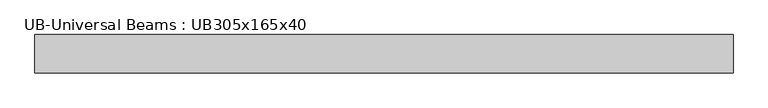
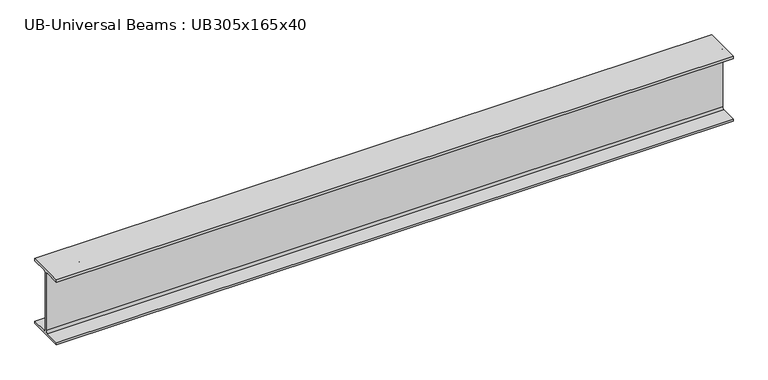
"""IFC4 building model written with IfcOpenShell, lengths in millimetres: beam geometry, UB-Universal Beams : UB305x165x40."""

from ifc_helpers import new_model, si_unit, point, frame, frame_2d, origin, place, context, project, spatial, polyline, circle_curve, trimmed, segment, composite_curve, outline, extrude, source, transform, mapped, element, save


def ub_universal_beams_ub305x165x40_59e17645(model_context):
    return source(origin(), model_context, "Body", "SweptSolid", [
        extrude(outline(composite_curve([segment(polyline([(82.5, -141.5), (82.5, -151.7), (-82.5, -151.7), (-82.5, -141.5), (-11.9, -141.5)]), True, "CONTINUOUS"), segment(trimmed(circle_curve(frame_2d((-11.9, -132.6)), 8.9), [point((-11.9, -141.5))], [point((-3.0, -132.6))], True, "CARTESIAN"), True, "CONTINUOUS"), segment(polyline([(-3.0, -132.6), (-3.0, 132.6)]), True, "CONTINUOUS"), segment(trimmed(circle_curve(frame_2d((-11.9, 132.6)), 8.9), [point((-3.0, 132.6))], [point((-11.9, 141.5))], True, "CARTESIAN"), True, "CONTINUOUS"), segment(polyline([(-11.9, 141.5), (-82.5, 141.5), (-82.5, 151.7), (82.5, 151.7), (82.5, 141.5), (11.9, 141.5)]), True, "CONTINUOUS"), segment(trimmed(circle_curve(frame_2d((11.9, 132.6)), 8.9), [point((11.9, 141.5))], [point((3.0, 132.6))], True, "CARTESIAN"), True, "CONTINUOUS"), segment(polyline([(3.0, 132.6), (3.0, -132.6)]), True, "CONTINUOUS"), segment(trimmed(circle_curve(frame_2d((11.9, -132.6)), 8.9), [point((3.0, -132.6))], [point((11.9, -141.5))], True, "CARTESIAN"), True, "CONTINUOUS"), segment(polyline([(11.9, -141.5), (82.5, -141.5)]), True, "CONTINUOUS")], self_intersect=False)), frame((-1500.0, 0.0, 0.0), z_axis=(1.0, 0.0, 0.0), x_axis=(0.0, 1.0, 0.0)), (0.0, 0.0, 1.0), 2987.2),
    ])


if __name__ == "__main__":
    model = new_model("IFC4")
    model_context = context("Model", 3, world=origin())
    ifc_project = project(units=[si_unit("LENGTHUNIT", "METRE", prefix="MILLI")], contexts=[model_context])
    site = spatial("IfcSite", under=ifc_project)
    building = spatial("IfcBuilding", under=site)
    placement = place(None, origin())
    ub_universal_beams_ub305x165x40_shape = ub_universal_beams_ub305x165x40_59e17645(model_context)
    element("IfcBeam", 1, ObjectType="UB-Universal Beams : UB305x165x40", at=placement, inside=building, context=model_context, shape_type="MappedRepresentation", body=[
        mapped(ub_universal_beams_ub305x165x40_shape, transform((0.0, 0.0, 0.0), x_axis=(1.0, 0.0, 0.0), y_axis=(0.0, 1.0, 0.0), z_axis=(0.0, 0.0, 1.0))),
    ])
    save(model, "model.ifc")

# Revit data of these elements
# Type "UB-Universal Beams : UB305x165x40"
#   Section Name Key = "UB305X165X40"
#   Width = 16.5 cm
#   Web Thickness = 0.6 cm
#   Web Fillet = 0.89 cm
#   Warping Constant = 164000.0 cm⁶
#   Torsional Moment of Inertia = 14.70 cm⁴
#   Section Area = 51.3 cm²
#   Plastic Modulus weak axis = 142.0 cm³
#   Plastic Modulus strong axis = 623.0 cm³
#   Nominal Weight = 40.2999 kgf/m
#   Moment of Inertia weak axis = 764.00 cm⁴
#   Moment of Inertia strong axis = 8503.00 cm⁴
#   Height = 30.34 cm
#   Flange Thickness = 1.02 cm
#   Elastic Modulus weak axis = 92.6 cm³
#   Elastic Modulus strong axis = 560.0 cm³
#   Centroid Vertical = 15.17 cm
#   Centroid Horizontal = 8.25 cm
#   Bolt Spacing = 9.0 cm
#   Length [instance default] = 1.5 m
#   Structural Material [instance default] = Metal - Steel 43-275
#   Type Comments = ""
#   Assembly Code = ""
# Element 1 (IfcBeam, "UB-Universal Beams : UB305x165x40")
#   Materials on its faces: "Metal - Steel 43-275"
# Materials
#   "Metal - Steel 43-275": class "Metal", colour RGB 247 247 247, transparency 0, Cost = 0
